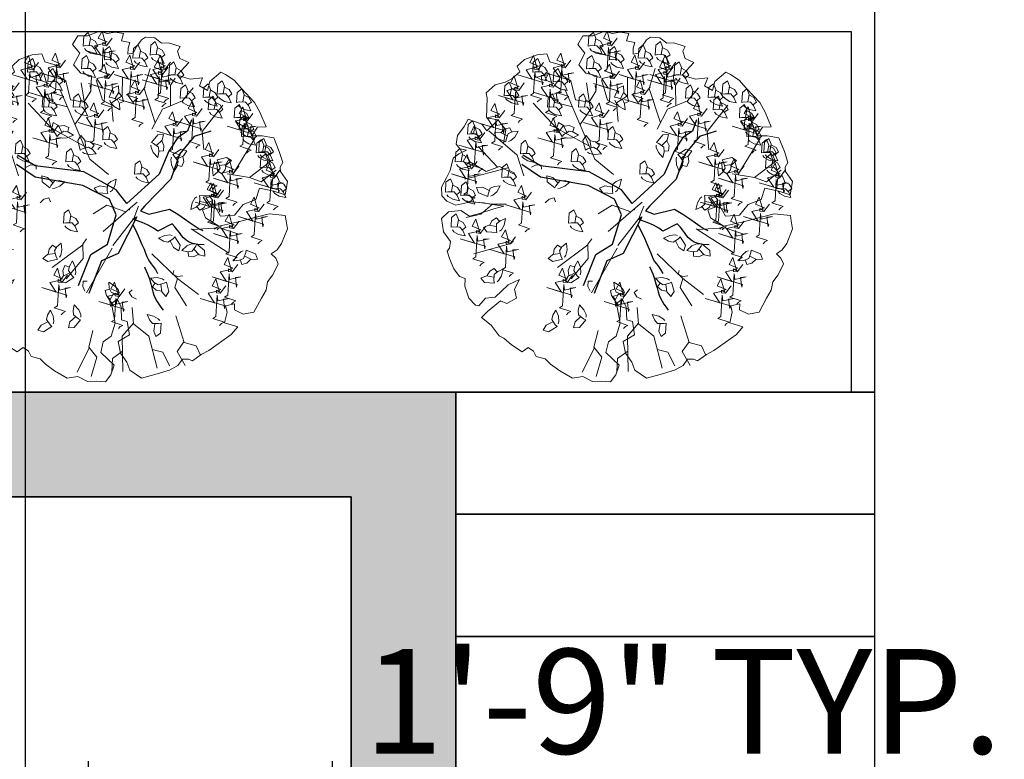
# Model space of a CAD drawing. Units: inches. Extents: x 2831 to 4250, y 1103 to 1797.
# Tile 12 of 15: x 3730 to 3814, y 1658 to 1722. Entities that reach past the tile are written whole.
import ezdxf

# ---------------------------------------------------------------- set-up
doc = ezdxf.new("R2010")
doc.units = ezdxf.units.IN
for name, color, linetype, lineweight in [('A-ANNO-DIMS', 2, 'Continuous', 18), ('A-WALL', 7, 'Continuous', 35), ('A-WALL-PATT', 252, 'Continuous', 13), ('ARBOL', 30, 'Continuous', 13), ('C-PROP', 7, 'Continuous', 25)]:
    doc.layers.add(name, color=color, linetype=linetype, lineweight=lineweight)
doc.layers.add('TALLO', color=36, linetype='Continuous')
doc.styles.get("Standard").update_dxf_attribs({"font": 'arial.ttf'})
doc.dimstyles.new('ISO-25', dxfattribs={"dimtxt": 9, "dimasz": 2.5, "dimexe": 1.25, "dimexo": 0.625, "dimtad": 1, "dimdec": 1, "dimlunit": 3, "dimtxsty": 'Standard', "dimcen": 2.5, "dimadec": 0, "dimazin": 0, "dimtfac": 1, "dimtdec": 1, "dimtmove": 0, "dimatfit": 3, "dimfxl": 1, "dimarcsym": 0})

# ---------------------------------------------------------------- blocks, each defined once
blk = doc.blocks.new('fresno')
at = {"layer": 'ARBOL'}
for p, q in [((2.96, 0.991), (3.575, 1.984)), ((-3.638, 1.194), (-4.164, 1.76)), ((-1.151, -0.932), (-1.99, -1.556)), ((-0.974, -3.757), (-1.31, -4.423))]:
    blk.add_line(p, q, dxfattribs=at)
blk.add_lwpolyline([(0.823, 4.745), (0.566, 4.764), (0.459, 4.687), (0.336, 4.518), (0.233, 4.322), (0.087, 4.298), (0.091, 4.464), (0.14, 4.621), (-0.09, 4.659), (-0.033, 4.863), (-0.264, 4.901), (-0.483, 4.866), (-0.686, 4.924), (-1.021, 4.801), (-1.288, 4.8), (-1.431, 4.563), (-1.234, 4.327), (-1.406, 4), (-1.205, 3.778), (-0.909, 3.705), (-0.931, 3.283), (-1.122, 2.983), (-1.491, 3.043), (-1.619, 3.562), (-1.9, 3.727), (-1.851, 3.982), (-2.197, 4.084), (-2.278, 4.31), (-2.543, 4.283), (-2.896, 4.152), (-3.091, 3.971), (-3.022, 3.817), (-3.244, 3.617), (-3.424, 3.528), (-3.697, 3.455), (-3.946, 3.236), (-3.922, 3.09), (-3.94, 2.548), (-3.617, 2.495), (-3.927, 2.19), (-4.062, 2.379), (-4.443, 2.512), (-4.546, 2.316), (-4.73, 2.062), (-4.767, 1.832), (-4.671, 1.698), (-4.486, 1.667), (-4.693, 1.559), (-4.854, 1.444), (-4.934, 1.102), (-5.037, 0.905), (-5.175, 0.644), (-5.166, 0.406), (-5.024, 0.264), (-4.781, 0.153), (-4.363, 0.249), (-4.014, 0.215), (-3.783, 0.177), (-3.46, 0.124), (-3.733, 0.051), (-4.132, -0.073), (-4.404, -0.146), (-4.639, 0.011), (-4.977, -0.028), (-5.172, -0.209), (-5.113, -0.574), (-4.921, -0.843), (-4.951, -1.027), (-5.012, -1.112), (-4.95, -1.311), (-4.83, -1.592), (-4.676, -1.807), (-4.518, -1.856), (-4.529, -2.068), (-4.417, -2.394), (-4.236, -2.59), (-4.143, -2.605), (-3.967, -2.397), (-3.703, -2.37), (-3.339, -2.027), (-3.032, -1.889), (-3.169, -2.15), (-3.115, -2.396), (-3.376, -2.542), (-3.552, -2.466), (-3.909, -2.762), (-4.077, -2.924), (-3.804, -3.135), (-3.592, -3.43), (-3.461, -3.499), (-3.253, -3.676), (-2.953, -3.867), (-2.792, -3.752), (-2.642, -3.848), (-2.572, -4.001), (-2.323, -4.066), (-2.18, -4.208), (-1.926, -4.392), (-1.58, -4.591), (-1.288, -4.545), (-1.027, -4.683), (-0.788, -4.675), (-0.531, -4.693), (-0.382, -4.505), (-0.29, -4.236), (-0.66, -3.891), (-0.588, -3.595), (-0.374, -3.441), (-0.267, -3.079), (-0.368, -2.541), (-0.208, -2.426), (-0.099, -2.633), (-0.087, -2.991), (0.071, -3.04), (0.129, -3.405), (-0.185, -3.59), (-0.119, -3.909), (0.055, -4.151), (0.136, -4.377), (0.456, -4.596), (0.828, -4.491), (1.227, -4.368), (1.461, -4.241), (1.583, -4.071), (1.748, -4.075), (1.86, -4.117), (2.101, -3.944), (2.308, -3.836), (2.925, -3.393), (3.101, -3.185), (2.74, -3.078), (2.812, -2.782), (2.769, -2.61), (3.015, -2.555), (3.012, -2.721), (3.254, -2.832), (3.546, -2.785), (3.752, -2.393), (3.882, -2.177), (3.92, -1.947), (4.069, -1.758), (4.214, -1.451), (4.144, -1.297), (4.021, -1.182), (4.182, -1.067), (4.304, -0.897), (4.464, -0.497), (4.429, -0.279), (4.406, -0.133), (3.964, -0.083), (3.074, -0.315), (2.582, -0.424), (2.217, -0.197), (2.136, 0.029), (2.462, 0.141), (2.628, -0.147), (3.012, -0.116), (3.249, 0.177), (3.602, 0.308), (3.701, 0.623), (4.089, 0.535), (4.404, 0.436), (4.464, 0.805), (4.272, 1.074), (4.267, 1.193), (4.336, 1.324), (4.243, 1.623), (4.092, 2.003), (3.769, 2.057), (3.485, 2.056), (3.642, 2.291), (3.88, 2.299), (3.71, 2.706), (3.563, 2.967), (3.201, 3.358), (3.001, 3.581), (2.766, 3.738), (2.635, 3.807), (2.332, 3.549), (2.268, 3.299), (2.052, 3.429), (2.136, 3.652), (1.798, 3.613), (1.437, 3.72), (1.755, 4.071), (1.513, 4.182), (1.451, 4.381), (1.519, 4.512), (1.204, 4.611), (1.012, 4.596)], close=True, dxfattribs=at)
for points in [[(-1.104, 4.45), (-1.063, 4.399), (-0.939, 4.325), (-0.757, 4.285), (-0.82, 4.431), (-0.903, 4.527), (-1.075, 4.533), (-1.143, 4.521), (-1.126, 4.792), (-1.002, 4.891), (-0.939, 4.738), (-0.975, 4.535)], [(-0.346, 4.735), (-0.501, 4.528), (-0.605, 4.545), (-0.605, 4.614), (-0.519, 4.563), (-0.622, 4.925), (-0.726, 4.735), (-0.484, 4.632), (-0.622, 4.58), (-0.829, 4.528), (-0.657, 4.27), (-1.053, 4.39), (-0.363, 4.183), (-0.381, 4.114), (-0.415, 4.373), (-0.26, 4.39), (-0.57, 4.321), (-0.588, 4.476), (-0.622, 3.89), (-0.708, 3.839), (-0.398, 3.735), (-0.467, 3.701), (-0.519, 3.649)], [(-0.935, 4.717), (-0.809, 4.65), (-0.736, 4.529), (-0.824, 4.459)], [(0.734, 4.203), (0.775, 4.152), (0.9, 4.078), (1.082, 4.038), (1.018, 4.185), (0.936, 4.281), (0.763, 4.287), (0.696, 4.274), (0.712, 4.546), (0.837, 4.645), (0.899, 4.491), (0.863, 4.289)], [(-0.521, 4.069), (-0.48, 4.018), (-0.356, 3.944), (-0.174, 3.904), (-0.237, 4.051), (-0.32, 4.146), (-0.492, 4.152), (-0.56, 4.14), (-0.543, 4.411), (-0.419, 4.511), (-0.356, 4.357), (-0.392, 4.154)], [(-0.352, 4.337), (-0.226, 4.269), (-0.153, 4.148), (-0.241, 4.078)], [(0.263, 4.114), (0.304, 4.063), (0.429, 3.989), (0.611, 3.948), (0.547, 4.095), (0.465, 4.191), (0.293, 4.197), (0.225, 4.185), (0.242, 4.456), (0.366, 4.555), (0.428, 4.402), (0.393, 4.199)], [(0.433, 4.381), (0.558, 4.314), (0.631, 4.193), (0.544, 4.122)], [(0.904, 4.471), (1.029, 4.404), (1.102, 4.282), (1.015, 4.212)], [(-2.368, 4.073), (-2.523, 3.866), (-2.627, 3.883), (-2.627, 3.952), (-2.541, 3.9), (-2.644, 4.262), (-2.748, 4.073), (-2.506, 3.969), (-2.644, 3.918), (-2.851, 3.866), (-2.679, 3.607), (-3.075, 3.728), (-2.385, 3.521), (-2.403, 3.452), (-2.437, 3.711), (-2.282, 3.728), (-2.592, 3.659), (-2.61, 3.814), (-2.644, 3.228), (-2.73, 3.176), (-2.42, 3.073), (-2.489, 3.038), (-2.541, 2.987)], [(-2.629, 3.733), (-2.588, 3.682), (-2.463, 3.608), (-2.281, 3.568), (-2.345, 3.715), (-2.427, 3.81), (-2.6, 3.816), (-2.667, 3.804), (-2.651, 4.075), (-2.526, 4.175), (-2.464, 4.021), (-2.5, 3.818)], [(-1.623, 4.132), (-1.778, 3.925), (-1.882, 3.942), (-1.882, 4.011), (-1.795, 3.959), (-1.899, 4.321), (-2.002, 4.132), (-1.761, 4.028), (-1.899, 3.977), (-2.106, 3.925), (-1.933, 3.666), (-2.33, 3.787), (-1.64, 3.58), (-1.657, 3.511), (-1.692, 3.77), (-1.537, 3.787), (-1.847, 3.718), (-1.864, 3.873), (-1.899, 3.287), (-1.985, 3.235), (-1.675, 3.132), (-1.744, 3.097), (-1.795, 3.046)], [(-1.149, 3.822), (-1.108, 3.771), (-0.983, 3.697), (-0.802, 3.657), (-0.865, 3.804), (-0.948, 3.9), (-1.12, 3.906), (-1.188, 3.893), (-1.171, 4.165), (-1.047, 4.264), (-0.984, 4.111), (-1.02, 3.908)], [(-0.98, 4.09), (-0.854, 4.023), (-0.781, 3.901), (-0.869, 3.831)], [(0.413, 4.08), (0.258, 3.873), (0.154, 3.89), (0.154, 3.959), (0.241, 3.908), (0.137, 4.27), (0.034, 4.08), (0.275, 3.977), (0.137, 3.925), (-0.07, 3.873), (0.103, 3.614), (-0.294, 3.735), (0.396, 3.528), (0.379, 3.459), (0.344, 3.718), (0.499, 3.735), (0.189, 3.666), (0.172, 3.821), (0.137, 3.235), (0.051, 3.183), (0.361, 3.08), (0.292, 3.046), (0.241, 2.994)], [(1.189, 3.942), (1.034, 3.735), (0.931, 3.752), (0.931, 3.821), (1.017, 3.77), (0.913, 4.132), (0.81, 3.942), (1.051, 3.839), (0.913, 3.787), (0.706, 3.735), (0.879, 3.477), (0.482, 3.597), (1.172, 3.39), (1.155, 3.321), (1.12, 3.58), (1.276, 3.597), (0.965, 3.528), (0.948, 3.683), (0.913, 3.097), (0.827, 3.046), (1.138, 2.942), (1.069, 2.908), (1.017, 2.856)], [(1.259, 4.08), (1.103, 3.873), (1, 3.89), (1, 3.959), (1.086, 3.908), (0.982, 4.27), (0.879, 4.08), (1.12, 3.977), (0.982, 3.925), (0.775, 3.873), (0.948, 3.614), (0.551, 3.735), (1.241, 3.528), (1.224, 3.459), (1.189, 3.718), (1.345, 3.735), (1.034, 3.666), (1.017, 3.821), (0.982, 3.235), (0.896, 3.183), (1.207, 3.08), (1.138, 3.046), (1.086, 2.994)], [(1.25, 3.643), (1.291, 3.592), (1.416, 3.518), (1.597, 3.478), (1.534, 3.625), (1.451, 3.721), (1.279, 3.727), (1.211, 3.714), (1.228, 3.985), (1.352, 4.085), (1.415, 3.931), (1.379, 3.729)], [(-1.951, 3.597), (-2.106, 3.39), (-2.209, 3.408), (-2.209, 3.477), (-2.123, 3.425), (-2.227, 3.787), (-2.33, 3.597), (-2.089, 3.494), (-2.227, 3.442), (-2.434, 3.39), (-2.261, 3.132), (-2.658, 3.252), (-1.968, 3.046), (-1.985, 2.977), (-2.02, 3.235), (-1.864, 3.252), (-2.175, 3.183), (-2.192, 3.339), (-2.227, 2.752), (-2.313, 2.701), (-2.002, 2.597), (-2.071, 2.563), (-2.123, 2.511)], [(-2.459, 4), (-2.334, 3.933), (-2.261, 3.812), (-2.348, 3.742)], [(-2.068, 3.464), (-2.027, 3.413), (-1.903, 3.339), (-1.721, 3.299), (-1.784, 3.446), (-1.867, 3.542), (-2.039, 3.547), (-2.107, 3.535), (-2.09, 3.806), (-1.966, 3.906), (-1.903, 3.752), (-1.939, 3.55)], [(-0.287, 3.833), (-0.442, 3.626), (-0.546, 3.643), (-0.546, 3.712), (-0.46, 3.661), (-0.563, 4.023), (-0.667, 3.833), (-0.425, 3.73), (-0.563, 3.678), (-0.77, 3.626), (-0.598, 3.367), (-0.995, 3.488), (-0.304, 3.281), (-0.322, 3.212), (-0.356, 3.471), (-0.201, 3.488), (-0.511, 3.419), (-0.529, 3.574), (-0.563, 2.988), (-0.649, 2.936), (-0.339, 2.833), (-0.408, 2.799), (-0.46, 2.747)], [(0.837, 2.414), (0.533, 3.352), (0.697, 3.906)], [(1.419, 3.911), (1.545, 3.844), (1.618, 3.722), (1.53, 3.652)], [(-2.898, 3.511), (-3.053, 3.304), (-3.157, 3.321), (-3.157, 3.39), (-3.071, 3.339), (-3.174, 3.701), (-3.278, 3.511), (-3.036, 3.408), (-3.174, 3.356), (-3.381, 3.304), (-3.209, 3.046), (-3.605, 3.166), (-2.915, 2.959), (-2.932, 2.89), (-2.967, 3.149), (-2.812, 3.166), (-3.122, 3.097), (-3.14, 3.253), (-3.174, 2.666), (-3.26, 2.615), (-2.95, 2.511), (-3.019, 2.477), (-3.071, 2.425)], [(-3.413, 3.083), (-3.373, 3.032), (-3.248, 2.958), (-3.066, 2.918), (-3.129, 3.065), (-3.212, 3.161), (-3.384, 3.167), (-3.452, 3.154), (-3.435, 3.425), (-3.311, 3.525), (-3.248, 3.371), (-3.284, 3.169)], [(-1.899, 3.732), (-1.773, 3.664), (-1.7, 3.543), (-1.788, 3.473)], [(-0.358, 2.895), (-0.615, 3.037), (-0.783, 3.596)], [(-0.063, 3.671), (-0.069, 3.151), (-0.364, 2.965), (-0.319, 2.449)], [(0.558, 3.402), (0.403, 3.195), (0.299, 3.212), (0.299, 3.281), (0.386, 3.23), (0.282, 3.592), (0.179, 3.402), (0.42, 3.299), (0.282, 3.247), (0.075, 3.195), (0.248, 2.936), (-0.149, 3.057), (0.541, 2.85), (0.524, 2.781), (0.489, 3.04), (0.644, 3.057), (0.334, 2.988), (0.317, 3.143), (0.282, 2.557), (0.196, 2.505), (0.506, 2.402), (0.437, 2.368), (0.386, 2.316)], [(1.259, 2.882), (1.254, 3.446), (1.381, 3.636)], [(2.573, 3.128), (2.613, 3.077), (2.738, 3.003), (2.92, 2.963), (2.857, 3.11), (2.774, 3.205), (2.602, 3.211), (2.534, 3.199), (2.551, 3.47), (2.675, 3.57), (2.738, 3.416), (2.702, 3.214)], [(-3.244, 3.351), (-3.118, 3.284), (-3.045, 3.162), (-3.133, 3.092)], [(-0.448, 1), (-0.961, 1.419), (-1.784, 3.341)], [(-1.367, 2.367), (-1.081, 2.78), (-1.193, 3.514)], [(-0.923, 3.449), (-0.951, 3.425), (-0.93, 3.313)], [(-0.41, 3.035), (-0.387, 2.974), (-0.291, 2.865), (-0.131, 2.771), (-0.146, 2.93), (-0.195, 3.047), (-0.357, 3.106), (-0.425, 3.115), (-0.325, 3.368), (-0.176, 3.424), (-0.164, 3.258), (-0.261, 3.077)], [(0.746, 2.242), (1.034, 2.786), (1.584, 3.019), (1.879, 3.374)], [(1.564, 3.016), (1.605, 2.965), (1.729, 2.891), (1.911, 2.851), (1.848, 2.998), (1.765, 3.094), (1.593, 3.099), (1.525, 3.087), (1.542, 3.358), (1.666, 3.458), (1.729, 3.304), (1.693, 3.102)], [(1.733, 3.284), (1.859, 3.216), (1.932, 3.095), (1.844, 3.025)], [(2.191, 3.038), (2.232, 2.987), (2.357, 2.913), (2.539, 2.873), (2.475, 3.02), (2.393, 3.116), (2.221, 3.122), (2.153, 3.109), (2.17, 3.381), (2.294, 3.48), (2.356, 3.326), (2.321, 3.124)], [(2.361, 3.306), (2.486, 3.239), (2.559, 3.117), (2.472, 3.047)], [(2.742, 3.396), (2.868, 3.328), (2.941, 3.207), (2.853, 3.137)], [(3.111, 2.904), (3.152, 2.853), (3.276, 2.779), (3.458, 2.739), (3.395, 2.886), (3.312, 2.981), (3.14, 2.987), (3.072, 2.975), (3.089, 3.246), (3.213, 3.346), (3.276, 3.192), (3.24, 2.99)], [(-2.225, 2.77), (-2.184, 2.718), (-2.06, 2.645), (-1.878, 2.604), (-1.941, 2.751), (-2.024, 2.847), (-2.196, 2.853), (-2.264, 2.84), (-2.247, 3.112), (-2.123, 3.211), (-2.06, 3.058), (-2.096, 2.855)], [(-1.575, 2.854), (-2.052, 2.969), (-2.2, 3.178)], [(-2.056, 3.037), (-1.93, 2.97), (-1.857, 2.849), (-1.945, 2.778)], [(-1.373, 2.77), (-1.332, 2.718), (-1.208, 2.645), (-1.026, 2.604), (-1.089, 2.751), (-1.172, 2.847), (-1.344, 2.853), (-1.412, 2.84), (-1.395, 3.112), (-1.271, 3.211), (-1.208, 3.058), (-1.244, 2.855)], [(-1.204, 3.037), (-1.078, 2.97), (-1.005, 2.849), (-1.093, 2.778)], [(-0.166, 3.238), (-0.068, 3.135), (-0.036, 2.997), (-0.141, 2.957)], [(2.121, 2.804), (1.966, 2.597), (1.862, 2.615), (1.862, 2.683), (1.949, 2.632), (1.845, 2.994), (1.742, 2.804), (1.983, 2.701), (1.845, 2.649), (1.638, 2.597), (1.811, 2.339), (1.414, 2.459), (2.104, 2.252), (2.087, 2.184), (2.052, 2.442), (2.207, 2.459), (1.897, 2.39), (1.88, 2.546), (1.845, 1.959), (1.759, 1.908), (2.069, 1.804), (2, 1.77), (1.949, 1.718)], [(2.326, 2.702), (2.367, 2.651), (2.492, 2.577), (2.673, 2.537), (2.61, 2.684), (2.527, 2.78), (2.355, 2.786), (2.287, 2.773), (2.304, 3.045), (2.428, 3.144), (2.491, 2.99), (2.455, 2.788)], [(3.28, 3.172), (3.406, 3.104), (3.479, 2.983), (3.391, 2.913)], [(-3.434, 2.752), (-3.59, 2.546), (-3.693, 2.563), (-3.693, 2.632), (-3.607, 2.58), (-3.71, 2.942), (-3.814, 2.752), (-3.572, 2.649), (-3.71, 2.597), (-3.917, 2.546), (-3.745, 2.287), (-4.142, 2.408), (-3.452, 2.201), (-3.469, 2.132), (-3.503, 2.39), (-3.348, 2.408), (-3.659, 2.339), (-3.676, 2.494), (-3.71, 1.908), (-3.797, 1.856), (-3.486, 1.753), (-3.555, 1.718), (-3.607, 1.666)], [(-1.112, 1.773), (-2.014, 2.265), (-2.654, 2.957)], [(-0.57, 2.77), (-0.726, 2.563), (-0.829, 2.58), (-0.829, 2.649), (-0.743, 2.597), (-0.846, 2.959), (-0.95, 2.77), (-0.708, 2.666), (-0.846, 2.615), (-1.053, 2.563), (-0.881, 2.304), (-1.278, 2.425), (-0.588, 2.218), (-0.605, 2.149), (-0.639, 2.408), (-0.484, 2.425), (-0.795, 2.356), (-0.812, 2.511), (-0.846, 1.925), (-0.933, 1.873), (-0.622, 1.77), (-0.691, 1.735), (-0.743, 1.684)], [(1.586, 2.528), (1.431, 2.321), (1.327, 2.339), (1.327, 2.408), (1.414, 2.356), (1.31, 2.718), (1.207, 2.528), (1.448, 2.425), (1.31, 2.373), (1.103, 2.321), (1.276, 2.063), (0.879, 2.184), (1.569, 1.977), (1.552, 1.908), (1.517, 2.166), (1.673, 2.184), (1.362, 2.115), (1.345, 2.27), (1.31, 1.684), (1.224, 1.632), (1.535, 1.528), (1.466, 1.494), (1.414, 1.442)], [(2.171, 1.674), (2.121, 2.172), (2.689, 2.898)], [(2.495, 2.97), (2.621, 2.903), (2.694, 2.781), (2.606, 2.711)], [(3.519, 2.666), (3.363, 2.459), (3.26, 2.477), (3.26, 2.546), (3.346, 2.494), (3.243, 2.856), (3.139, 2.666), (3.381, 2.563), (3.243, 2.511), (3.036, 2.459), (3.208, 2.201), (2.811, 2.321), (3.501, 2.115), (3.484, 2.046), (3.45, 2.304), (3.605, 2.321), (3.294, 2.252), (3.277, 2.408), (3.243, 1.821), (3.156, 1.77), (3.467, 1.666), (3.398, 1.632), (3.346, 1.58)], [(3.043, 2.478), (3.084, 2.427), (3.209, 2.353), (3.391, 2.313), (3.327, 2.46), (3.245, 2.556), (3.073, 2.562), (3.005, 2.549), (3.022, 2.82), (3.146, 2.92), (3.208, 2.766), (3.173, 2.564)], [(3.213, 2.746), (3.338, 2.679), (3.411, 2.557), (3.324, 2.487)], [(-4.422, 2.03), (-4.381, 1.979), (-4.257, 1.905), (-4.075, 1.865), (-4.138, 2.012), (-4.221, 2.108), (-4.393, 2.114), (-4.461, 2.101), (-4.444, 2.372), (-4.32, 2.472), (-4.257, 2.318), (-4.293, 2.116)], [(-3.468, 1.85), (-3.409, 2.222), (-3.628, 2.505)], [(-1.817, 2.351), (-1.972, 2.144), (-2.075, 2.162), (-2.075, 2.231), (-1.989, 2.179), (-2.093, 2.541), (-2.196, 2.351), (-1.955, 2.248), (-2.093, 2.196), (-2.3, 2.144), (-2.127, 1.886), (-2.524, 2.006), (-1.834, 1.8), (-1.851, 1.731), (-1.886, 1.989), (-1.73, 2.006), (-2.041, 1.937), (-2.058, 2.093), (-2.093, 1.506), (-2.179, 1.455), (-1.868, 1.351), (-1.937, 1.317), (-1.989, 1.265)], [(3.178, 2.165), (3.219, 2.113), (3.344, 2.04), (3.525, 1.999), (3.462, 2.146), (3.379, 2.242), (3.207, 2.248), (3.139, 2.236), (3.156, 2.507), (3.28, 2.606), (3.343, 2.453), (3.307, 2.25)], [(-3.986, 2.149), (-4.142, 1.942), (-4.245, 1.959), (-4.245, 2.028), (-4.159, 1.977), (-4.262, 2.339), (-4.366, 2.149), (-4.124, 2.046), (-4.262, 1.994), (-4.47, 1.942), (-4.297, 1.684), (-4.694, 1.804), (-4.004, 1.597), (-4.021, 1.528), (-4.055, 1.787), (-3.9, 1.804), (-4.211, 1.735), (-4.228, 1.89), (-4.262, 1.304), (-4.349, 1.253), (-4.038, 1.149), (-4.107, 1.115), (-4.159, 1.063)], [(-4.253, 2.298), (-4.127, 2.231), (-4.054, 2.109), (-4.142, 2.039)], [(-2.916, 0.958), (-3.096, 1.528), (-3.871, 2.197)], [(-3.331, 1.905), (-3.269, 1.928), (-3.161, 2.024), (-3.066, 2.184), (-3.226, 2.169), (-3.342, 2.121), (-3.401, 1.958), (-3.41, 1.89), (-3.663, 1.99), (-3.719, 2.139), (-3.554, 2.151), (-3.372, 2.054)], [(-3.533, 2.149), (-3.43, 2.247), (-3.292, 2.279), (-3.252, 2.174)], [(-1.786, 2.007), (-1.722, 1.99), (-1.578, 2.003), (-1.407, 2.078), (-1.545, 2.159), (-1.668, 2.188), (-1.811, 2.092), (-1.859, 2.042), (-2.004, 2.271), (-1.962, 2.425), (-1.821, 2.337), (-1.731, 2.152)], [(-1.806, 2.323), (-1.665, 2.343), (-1.534, 2.287), (-1.564, 2.179)], [(-0.566, 1.873), (-0.525, 1.822), (-0.4, 1.748), (-0.219, 1.708), (-0.282, 1.855), (-0.365, 1.951), (-0.537, 1.957), (-0.605, 1.944), (-0.588, 2.216), (-0.464, 2.315), (-0.401, 2.162), (-0.437, 1.959)], [(3.245, 1.963), (3.286, 1.912), (3.411, 1.838), (3.593, 1.798), (3.529, 1.945), (3.447, 2.041), (3.274, 2.046), (3.206, 2.034), (3.223, 2.305), (3.347, 2.405), (3.41, 2.251), (3.374, 2.049)], [(3.347, 2.432), (3.473, 2.365), (3.546, 2.244), (3.458, 2.173)], [(3.415, 2.231), (3.54, 2.163), (3.613, 2.042), (3.525, 1.972)], [(-2.965, 1.493), (-2.924, 1.441), (-2.799, 1.368), (-2.618, 1.327), (-2.681, 1.474), (-2.764, 1.57), (-2.936, 1.576), (-3.004, 1.564), (-2.987, 1.835), (-2.863, 1.934), (-2.8, 1.781), (-2.836, 1.578)], [(-1.164, 1.612), (-1.109, 1.576), (-0.967, 1.544), (-0.782, 1.562), (-0.888, 1.682), (-0.996, 1.748), (-1.162, 1.7), (-1.222, 1.667), (-1.29, 1.93), (-1.203, 2.063), (-1.096, 1.937), (-1.067, 1.733)], [(-1.085, 1.919), (-0.945, 1.893), (-0.838, 1.801), (-0.9, 1.707)], [(-0.397, 2.141), (-0.271, 2.074), (-0.198, 1.952), (-0.286, 1.882)], [(0.72, 1.798), (0.723, 1.733), (0.781, 1.6), (0.904, 1.46), (0.939, 1.616), (0.929, 1.742), (0.793, 1.848), (0.73, 1.878), (0.904, 2.088), (1.062, 2.095), (1.023, 1.934), (0.875, 1.791)], [(1.014, 1.915), (1.077, 1.787), (1.064, 1.646), (0.952, 1.64)], [(3.649, 1.515), (3.69, 1.464), (3.814, 1.39), (3.996, 1.35), (3.933, 1.497), (3.85, 1.592), (3.678, 1.598), (3.61, 1.586), (3.627, 1.857), (3.751, 1.957), (3.814, 1.803), (3.778, 1.601)], [(3.716, 1.537), (3.757, 1.486), (3.882, 1.412), (4.063, 1.372), (4, 1.519), (3.917, 1.615), (3.745, 1.621), (3.677, 1.608), (3.694, 1.88), (3.818, 1.979), (3.881, 1.825), (3.845, 1.623)], [(-4.759, 1.269), (-4.718, 1.217), (-4.593, 1.144), (-4.411, 1.103), (-4.475, 1.25), (-4.557, 1.346), (-4.729, 1.352), (-4.797, 1.339), (-4.78, 1.611), (-4.656, 1.71), (-4.594, 1.557), (-4.629, 1.354)], [(-2.796, 1.76), (-2.67, 1.693), (-2.597, 1.572), (-2.685, 1.501)], [(-1.575, 1.269), (-1.534, 1.217), (-1.409, 1.144), (-1.228, 1.103), (-1.291, 1.25), (-1.373, 1.346), (-1.546, 1.352), (-1.614, 1.339), (-1.597, 1.611), (-1.473, 1.71), (-1.41, 1.557), (-1.446, 1.354)], [(1.283, 1.469), (1.266, 1.405), (1.279, 1.261), (1.354, 1.09), (1.435, 1.228), (1.464, 1.351), (1.368, 1.494), (1.318, 1.542), (1.547, 1.687), (1.7, 1.645), (1.613, 1.504), (1.428, 1.414)], [(2.587, 1.684), (2.432, 1.477), (2.328, 1.494), (2.328, 1.563), (2.414, 1.511), (2.311, 1.873), (2.207, 1.684), (2.449, 1.58), (2.311, 1.528), (2.104, 1.477), (2.276, 1.218), (1.88, 1.339), (2.57, 1.132), (2.552, 1.063), (2.518, 1.321), (2.673, 1.339), (2.363, 1.27), (2.345, 1.425), (2.311, 0.839), (2.225, 0.787), (2.535, 0.684), (2.466, 0.649), (2.414, 0.597)], [(3.818, 1.783), (3.944, 1.715), (4.017, 1.594), (3.929, 1.524)], [(3.885, 1.805), (4.011, 1.738), (4.084, 1.616), (3.996, 1.546)], [(-4.193, 1.356), (-4.349, 1.149), (-4.452, 1.166), (-4.452, 1.235), (-4.366, 1.184), (-4.469, 1.546), (-4.573, 1.356), (-4.331, 1.253), (-4.469, 1.201), (-4.677, 1.149), (-4.504, 0.89), (-4.901, 1.011), (-4.211, 0.804), (-4.228, 0.735), (-4.262, 0.994), (-4.107, 1.011), (-4.418, 0.942), (-4.435, 1.097), (-4.469, 0.511), (-4.556, 0.459), (-4.245, 0.356), (-4.314, 0.322), (-4.366, 0.27)], [(-4.589, 1.536), (-4.464, 1.469), (-4.391, 1.348), (-4.478, 1.277)], [(-1.406, 1.536), (-1.28, 1.469), (-1.207, 1.348), (-1.295, 1.277)], [(0.308, 0.933), (0.349, 0.881), (0.474, 0.807), (0.656, 0.767), (0.592, 0.914), (0.51, 1.01), (0.337, 1.016), (0.27, 1.003), (0.286, 1.275), (0.411, 1.374), (0.473, 1.221), (0.437, 1.018)], [(1.599, 1.489), (1.618, 1.348), (1.563, 1.217), (1.455, 1.247)], [(2.479, 1.34), (2.443, 1.285), (2.411, 1.143), (2.429, 0.958), (2.549, 1.064), (2.615, 1.172), (2.567, 1.338), (2.534, 1.398), (2.797, 1.466), (2.93, 1.379), (2.804, 1.272), (2.6, 1.243)], [(3.139, 1.235), (2.984, 1.028), (2.88, 1.046), (2.88, 1.115), (2.967, 1.063), (2.863, 1.425), (2.759, 1.235), (3.001, 1.132), (2.863, 1.08), (2.656, 1.028), (2.828, 0.77), (2.432, 0.891), (3.122, 0.684), (3.105, 0.615), (3.07, 0.873), (3.225, 0.891), (2.915, 0.822), (2.897, 0.977), (2.863, 0.391), (2.777, 0.339), (3.087, 0.235), (3.018, 0.201), (2.967, 0.149)], [(4.01, 1.36), (3.422, 0.918)], [(3.761, 1.112), (3.802, 1.061), (3.926, 0.987), (4.108, 0.947), (4.045, 1.093), (3.962, 1.189), (3.79, 1.195), (3.722, 1.183), (3.739, 1.454), (3.863, 1.553), (3.926, 1.4), (3.89, 1.197)], [(3.93, 1.379), (4.056, 1.312), (4.129, 1.191), (4.041, 1.121)], [(-3.354, 1.176), (-4.529, 0.864)], [(-3.192, 1.017), (-3.578, 1.215), (-3.949, 1.081), (-4.398, 1.339)], [(-3.481, 0.843), (-3.44, 0.792), (-3.315, 0.718), (-3.133, 0.678), (-3.197, 0.825), (-3.279, 0.92), (-3.451, 0.926), (-3.519, 0.914), (-3.502, 1.185), (-3.378, 1.285), (-3.316, 1.131), (-3.351, 0.928)], [(-3.311, 1.111), (-3.186, 1.043), (-3.113, 0.922), (-3.2, 0.852)], [(-2.703, 1.201), (-2.575, 1.263), (-2.433, 1.251), (-2.428, 1.139)], [(0.478, 1.2), (0.603, 1.133), (0.676, 1.011), (0.589, 0.941)], [(2.786, 1.261), (2.76, 1.121), (2.668, 1.014), (2.574, 1.076)], [(2.808, 1.015), (3.422, 0.918), (3.422, 0.918), (3.748, 0.794), (4.154, 1.111)], [(4.26, 1.115), (4.105, 0.908), (4.002, 0.925), (4.002, 0.994), (4.088, 0.942), (3.984, 1.304), (3.881, 1.115), (4.122, 1.011), (3.984, 0.959), (3.777, 0.908), (3.95, 0.649), (3.553, 0.77), (4.243, 0.563), (4.226, 0.494), (4.191, 0.753), (4.347, 0.77), (4.036, 0.701), (4.019, 0.856), (3.984, 0.27), (3.898, 0.218), (4.209, 0.115), (4.14, 0.08), (4.088, 0.029)], [(-5.028, 0.44), (-4.987, 0.388), (-4.862, 0.315), (-4.68, 0.274), (-4.744, 0.421), (-4.826, 0.517), (-4.998, 0.523), (-5.066, 0.511), (-5.049, 0.782), (-4.925, 0.881), (-4.863, 0.728), (-4.898, 0.525)], [(-1.981, 0.615), (-1.915, 0.618), (-1.782, 0.676), (-1.643, 0.799), (-1.799, 0.834), (-1.925, 0.824), (-2.031, 0.688), (-2.061, 0.626), (-2.27, 0.799), (-2.278, 0.958), (-2.117, 0.918), (-1.974, 0.77)], [(-0.397, 0.517), (-0.346, 0.557), (-0.272, 0.682), (-0.232, 0.864), (-0.379, 0.801), (-0.474, 0.718), (-0.48, 0.546), (-0.468, 0.478), (-0.739, 0.495), (-0.838, 0.619), (-0.685, 0.682), (-0.482, 0.646)], [(4.075, 0.529), (4.116, 0.478), (4.24, 0.404), (4.422, 0.364), (4.359, 0.511), (4.276, 0.607), (4.104, 0.613), (4.036, 0.6), (4.053, 0.871), (4.177, 0.971), (4.24, 0.817), (4.204, 0.615)], [(-4.858, 0.707), (-4.733, 0.64), (-4.66, 0.519), (-4.747, 0.448)], [(-4.602, 0.35), (-4.561, 0.299), (-4.436, 0.225), (-4.254, 0.185), (-4.318, 0.332), (-4.4, 0.428), (-4.572, 0.433), (-4.64, 0.421), (-4.623, 0.692), (-4.499, 0.792), (-4.437, 0.638), (-4.472, 0.436)], [(-4.432, 0.618), (-4.307, 0.55), (-4.234, 0.429), (-4.321, 0.359)], [(-3.824, 0.404), (-3.763, 0.427), (-3.654, 0.523), (-3.559, 0.683), (-3.719, 0.668), (-3.835, 0.62), (-3.894, 0.457), (-3.903, 0.389), (-4.156, 0.489), (-4.212, 0.638), (-4.047, 0.65), (-3.865, 0.553)], [(-2.698, 0.509), (-2.854, 0.302), (-2.957, 0.319), (-2.957, 0.388), (-2.871, 0.336), (-2.974, 0.698), (-3.078, 0.509), (-2.836, 0.405), (-2.974, 0.353), (-3.182, 0.302), (-3.009, 0.043), (-3.406, 0.164), (-2.716, -0.043), (-2.733, -0.112), (-2.767, 0.147), (-2.612, 0.164), (-2.923, 0.095), (-2.94, 0.25), (-2.974, -0.336), (-3.061, -0.388), (-2.75, -0.491), (-2.819, -0.526), (-2.871, -0.577)], [(2.639, 0.58), (2.483, 0.373), (2.38, 0.391), (2.38, 0.46), (2.466, 0.408), (2.363, 0.77), (2.259, 0.58), (2.501, 0.477), (2.363, 0.425), (2.156, 0.373), (2.328, 0.115), (1.931, 0.235), (2.621, 0.029), (2.604, -0.04), (2.57, 0.218), (2.725, 0.235), (2.414, 0.166), (2.397, 0.322), (2.363, -0.265), (2.276, -0.316), (2.587, -0.42), (2.518, -0.454), (2.466, -0.506)], [(2.708, 0.563), (2.552, 0.356), (2.449, 0.373), (2.449, 0.442), (2.535, 0.391), (2.432, 0.753), (2.328, 0.563), (2.57, 0.46), (2.432, 0.408), (2.225, 0.356), (2.397, 0.097), (2, 0.218), (2.69, 0.011), (2.673, -0.058), (2.639, 0.201), (2.794, 0.218), (2.483, 0.149), (2.466, 0.304), (2.432, -0.282), (2.345, -0.334), (2.656, -0.437), (2.587, -0.471), (2.535, -0.523)], [(4.244, 0.797), (4.37, 0.73), (4.443, 0.608), (4.355, 0.538)], [(-2.322, 0.222), (-2.219, 0.321), (-2.081, 0.353), (-2.042, 0.248)], [(1.978, 0.384), (1.927, 0.343), (1.853, 0.218), (1.813, 0.036), (1.96, 0.1), (2.056, 0.182), (2.061, 0.355), (2.049, 0.422), (2.32, 0.406), (2.42, 0.281), (2.266, 0.219), (2.064, 0.254)], [(3.829, 0.184), (3.674, -0.023), (3.57, -0.006), (3.57, 0.063), (3.657, 0.011), (3.553, 0.373), (3.45, 0.184), (3.691, 0.08), (3.553, 0.029), (3.346, -0.023), (3.519, -0.282), (3.122, -0.161), (3.812, -0.368), (3.795, -0.437), (3.76, -0.178), (3.915, -0.161), (3.605, -0.23), (3.588, -0.075), (3.553, -0.661), (3.467, -0.713), (3.777, -0.816), (3.708, -0.851), (3.657, -0.902)], [(-3.394, 0.18), (-3.77, 0.182), (-4.532, 0.27)], [(-3.77, 0.182), (-4.09, -0.088), (-4.494, -0.18)], [(-1.642, -0.412), (-1.601, -0.463), (-1.477, -0.537), (-1.295, -0.577), (-1.358, -0.43), (-1.441, -0.334), (-1.613, -0.328), (-1.681, -0.341), (-1.664, -0.069), (-1.54, 0.03), (-1.477, -0.124), (-1.513, -0.326)], [(0.03, -0.026), (-0.491, 0.154), (-0.871, -0.08)], [(-0.596, -0.564), (0.03, -0.026), (0.339, 0.235)], [(0.38, 0.131), (0.248, -0.21), (-0.33, -0.951)], [(2.246, 0.214), (2.178, 0.089), (2.057, 0.016), (1.987, 0.103)], [(-4.871, -0.524), (-4.83, -0.575), (-4.705, -0.649), (-4.523, -0.689), (-4.587, -0.542), (-4.669, -0.446), (-4.841, -0.44), (-4.909, -0.453), (-4.893, -0.181), (-4.768, -0.082), (-4.706, -0.236), (-4.741, -0.438)], [(-4.701, -0.256), (-4.576, -0.323), (-4.503, -0.445), (-4.59, -0.515)], [(-3.952, -0.42), (-4.107, -0.627), (-4.211, -0.609), (-4.211, -0.54), (-4.124, -0.592), (-4.228, -0.23), (-4.331, -0.42), (-4.09, -0.523), (-4.228, -0.575), (-4.435, -0.627), (-4.262, -0.885), (-4.659, -0.765), (-3.969, -0.971), (-3.986, -1.04), (-4.021, -0.782), (-3.866, -0.765), (-4.176, -0.834), (-4.193, -0.678), (-4.228, -1.265), (-4.314, -1.316), (-4.004, -1.42), (-4.073, -1.454), (-4.124, -1.506)], [(-3.58, -0.559), (-3.529, -0.518), (-3.455, -0.393), (-3.415, -0.211), (-3.562, -0.275), (-3.658, -0.357), (-3.664, -0.53), (-3.651, -0.597), (-3.923, -0.581), (-4.022, -0.456), (-3.868, -0.394), (-3.666, -0.43)], [(-3.848, -0.389), (-3.781, -0.264), (-3.659, -0.191), (-3.589, -0.278)], [(-1.473, -0.144), (-1.347, -0.211), (-1.274, -0.333), (-1.362, -0.403)], [(3.139, -0.282), (2.984, -0.489), (2.88, -0.471), (2.88, -0.402), (2.967, -0.454), (2.863, -0.092), (2.759, -0.282), (3.001, -0.385), (2.863, -0.437), (2.656, -0.489), (2.828, -0.747), (2.432, -0.627), (3.122, -0.834), (3.105, -0.902), (3.07, -0.644), (3.225, -0.627), (2.915, -0.696), (2.897, -0.54), (2.863, -1.127), (2.777, -1.178), (3.087, -1.282), (3.018, -1.316), (2.967, -1.368)], [(-3.141, -0.713), (-3.296, -0.92), (-3.4, -0.902), (-3.4, -0.834), (-3.314, -0.885), (-3.417, -0.523), (-3.521, -0.713), (-3.279, -0.816), (-3.417, -0.868), (-3.624, -0.92), (-3.452, -1.178), (-3.848, -1.058), (-3.158, -1.265), (-3.175, -1.333), (-3.21, -1.075), (-3.055, -1.058), (-3.365, -1.127), (-3.383, -0.971), (-3.417, -1.558), (-3.503, -1.609), (-3.193, -1.713), (-3.262, -1.747), (-3.314, -1.799)], [(1.822, -0.495), (2.859, -1.165)], [(1.846, -0.51), (2.605, -0.469), (3.129, -0.637)], [(-1.047, -0.767), (-1.151, -0.913), (-1.144, -1.307), (-1.61, -1.871)], [(1.304, -0.681), (1.241, -0.664), (1.097, -0.678), (0.926, -0.752), (1.064, -0.833), (1.187, -0.862), (1.33, -0.766), (1.377, -0.716), (1.523, -0.945), (1.481, -1.099), (1.34, -1.011), (1.25, -0.826)], [(-3.195, -0.824), (-3.267, -0.898), (-4.285, -1.185)], [(-1.794, -1.268), (-1.758, -1.214), (-1.726, -1.072), (-1.744, -0.887), (-1.865, -0.993), (-1.93, -1.101), (-1.883, -1.266), (-1.85, -1.327), (-2.113, -1.395), (-2.246, -1.307), (-2.119, -1.2), (-1.916, -1.172)], [(-2.101, -1.19), (-2.076, -1.05), (-1.983, -0.943), (-1.889, -1.004)], [(-0.346, -1.024), (-1.05, -2.251)], [(1.903, -0.903), (1.837, -0.905), (1.704, -0.963), (1.565, -1.086), (1.721, -1.122), (1.847, -1.111), (1.953, -0.975), (1.983, -0.913), (2.192, -1.086), (2.2, -1.245), (2.039, -1.205), (1.896, -1.057)], [(3.253, -1.094), (3.192, -1.117), (3.083, -1.213), (2.988, -1.374), (3.148, -1.359), (3.264, -1.31), (3.323, -1.148), (3.332, -1.079), (3.585, -1.179), (3.641, -1.328), (3.476, -1.34), (3.294, -1.244)], [(0.748, -1.185), (1.452, -1.855), (2.021, -2.292)], [(2.02, -1.197), (1.891, -1.259), (1.75, -1.247), (1.745, -1.134)], [(3.105, -1.471), (2.949, -1.678), (2.846, -1.661), (2.846, -1.592), (2.932, -1.644), (2.829, -1.282), (2.725, -1.471), (2.967, -1.575), (2.829, -1.627), (2.621, -1.678), (2.794, -1.937), (2.397, -1.816), (3.087, -2.023), (3.07, -2.092), (3.036, -1.833), (3.191, -1.816), (2.88, -1.885), (2.863, -1.73), (2.829, -2.316), (2.742, -2.368), (3.053, -2.471), (2.984, -2.506), (2.932, -2.558)], [(3.455, -1.338), (3.352, -1.437), (3.214, -1.469), (3.175, -1.364)], [(-3.648, -1.948), (-3.596, -1.907), (-3.523, -1.782), (-3.482, -1.6), (-3.629, -1.664), (-3.725, -1.746), (-3.731, -1.919), (-3.719, -1.986), (-3.99, -1.97), (-4.089, -1.845), (-3.936, -1.783), (-3.733, -1.819)], [(-3.915, -1.778), (-3.848, -1.653), (-3.727, -1.58), (-3.656, -1.667)], [(-1.571, -1.764), (-1.726, -1.971), (-1.83, -1.954), (-1.83, -1.885), (-1.744, -1.937), (-1.847, -1.575), (-1.951, -1.764), (-1.709, -1.868), (-1.847, -1.92), (-2.054, -1.971), (-1.882, -2.23), (-2.278, -2.109), (-1.588, -2.316), (-1.605, -2.385), (-1.64, -2.127), (-1.485, -2.109), (-1.795, -2.178), (-1.813, -2.023), (-1.847, -2.609), (-1.933, -2.661), (-1.623, -2.764), (-1.692, -2.799), (-1.744, -2.851)], [(-1.361, -1.756), (-1.343, -1.693), (-1.357, -1.548), (-1.431, -1.377), (-1.513, -1.515), (-1.542, -1.638), (-1.445, -1.781), (-1.395, -1.829), (-1.625, -1.974), (-1.778, -1.932), (-1.691, -1.791), (-1.506, -1.701)], [(-1.677, -1.776), (-1.696, -1.635), (-1.641, -1.504), (-1.533, -1.534)], [(1.086, -1.899), (1.031, -1.863), (0.89, -1.831), (0.704, -1.849), (0.81, -1.969), (0.918, -2.035), (1.084, -1.987), (1.145, -1.954), (1.212, -2.218), (1.125, -2.35), (1.018, -2.224), (0.989, -2.02)], [(1.593, -1.781), (1.452, -1.801), (1.322, -1.746), (1.352, -1.637)], [(1.452, -1.855), (1.379, -2.105), (1.698, -2.609)], [(2.777, -2.058), (2.621, -2.264), (2.518, -2.247), (2.518, -2.178), (2.604, -2.23), (2.501, -1.868), (2.397, -2.058), (2.639, -2.161), (2.501, -2.213), (2.294, -2.264), (2.466, -2.523), (2.069, -2.402), (2.759, -2.609), (2.742, -2.678), (2.708, -2.42), (2.863, -2.402), (2.552, -2.471), (2.535, -2.316), (2.501, -2.902), (2.414, -2.954), (2.725, -3.057), (2.656, -3.092), (2.604, -3.144)], [(-1.092, -2.202), (-1.154, -2.074), (-1.142, -1.933), (-1.03, -1.928)], [(-0.001, -2.144), (-0.156, -2.351), (-0.26, -2.333), (-0.26, -2.264), (-0.174, -2.316), (-0.277, -1.954), (-0.381, -2.144), (-0.139, -2.247), (-0.277, -2.299), (-0.484, -2.351), (-0.312, -2.609), (-0.708, -2.489), (-0.018, -2.695), (-0.035, -2.764), (-0.07, -2.506), (0.085, -2.489), (-0.225, -2.558), (-0.243, -2.402), (-0.277, -2.989), (-0.363, -3.04), (-0.053, -3.144), (-0.122, -3.178), (-0.174, -3.23)], [(-0.405, -2.427), (-0.503, -2.324), (-0.535, -2.186), (-0.43, -2.146)], [(-0.161, -2.225), (-0.184, -2.163), (-0.28, -2.055), (-0.44, -1.96), (-0.425, -2.12), (-0.376, -2.236), (-0.214, -2.295), (-0.146, -2.304), (-0.246, -2.557), (-0.395, -2.613), (-0.407, -2.448), (-0.31, -2.266)], [(1.007, -2.206), (0.867, -2.181), (0.76, -2.088), (0.822, -1.994)], [(0.319, -2.428), (0.193, -2.361), (0.12, -2.239), (0.208, -2.169)], [(-1.201, -2.914), (-1.204, -2.849), (-1.262, -2.716), (-1.385, -2.576), (-1.42, -2.732), (-1.41, -2.858), (-1.274, -2.964), (-1.212, -2.994), (-1.385, -3.204), (-1.544, -3.211), (-1.504, -3.05), (-1.356, -2.907)], [(0.201, -2.655), (0.24, -3.105), (0.657, -3.436), (0.886, -4.322)], [(-1.966, -3.1), (-1.949, -3.037), (-1.962, -2.892), (-2.037, -2.722), (-2.118, -2.859), (-2.147, -2.982), (-2.051, -3.125), (-2.001, -3.173), (-2.23, -3.319), (-2.383, -3.277), (-2.296, -3.136), (-2.111, -3.046)], [(0.959, -3.012), (0.918, -2.961), (0.793, -2.887), (0.612, -2.847), (0.675, -2.994), (0.758, -3.089), (0.93, -3.095), (0.998, -3.083), (0.981, -3.354), (0.857, -3.453), (0.794, -3.3), (0.83, -3.097)], [(1.399, -2.886), (1.63, -3.612), (1.964, -3.708), (2.084, -3.964)], [(0.238, -3.084), (-0.067, -3.438), (-0.048, -4.412)], [(-0.923, -4.549), (-0.768, -4.012), (-0.99, -3.737), (-0.872, -3.28)], [(1.625, -3.596), (1.438, -3.858), (1.657, -4.248)], [(-0.059, -3.851), (-0.336, -4.054), (-0.355, -4.41)], [(0.752, -3.801), (1.042, -3.878), (1.233, -4.25)]]:
    blk.add_lwpolyline(points, dxfattribs=at)
for p in [(-0.308, 0.101), (0.124, 0.027)]:
    blk.add_point(p, dxfattribs=at)
at = {"layer": 'TALLO'}
for points in [[(1.829, 2.5), (1.722, 2.184), (1.454, 2.012), (1.213, 1.639), (0.944, 1.008), (0.06, 0.204), (-0.234, 0.577), (-1.119, 1.065), (-2.458, 1.237), (-2.941, 1.524)], [(2.364, 2.184), (1.909, 2.041), (1.507, 1.552), (1.266, 0.864), (0.542, 0.125), (0.433, 0.001), (0.662, -0.096), (1.228, 0.045), (1.455, -0.09), (1.644, -0.216), (1.8, -0.33), (1.931, -0.425), (2.042, -0.496), (2.141, -0.539)], [(-1.272, -2.047), (-0.931, -1.203), (-0.475, -0.916), (-0.234, -0.112), (-0.422, 0.318), (-1.146, 0.691), (-2.458, 0.921), (-2.967, 1.266)], [(2.177, -0.932), (2.008, -0.924), (1.873, -0.898), (1.766, -0.859), (1.682, -0.807), (1.613, -0.745), (1.554, -0.676), (1.499, -0.6), (1.442, -0.521), (1.376, -0.44), (1.298, -0.357), (0.908, -0.555), (0.791, -0.474), (0.647, -0.394), (0.474, -0.317), (0.265, -0.244), (0.226, -0.233), (0.328, -0.17), (-0.181, -1.175), (-0.637, -1.375), (-0.985, -2.265)], [(0.219, -0.386), (0.3, -0.544), (0.399, -0.753), (0.473, -0.922), (0.529, -1.057), (0.571, -1.164), (0.607, -1.251), (0.641, -1.324), (0.68, -1.389), (0.729, -1.454), (0.784, -1.525), (0.844, -1.61), (0.903, -1.717)], [(0.538, -1.536), (0.555, -1.568), (0.626, -1.728), (0.678, -1.871), (0.716, -2), (0.747, -2.115), (0.773, -2.219), (0.802, -2.314), (0.837, -2.401), (0.883, -2.483), (0.936, -2.562), (0.994, -2.642), (1.052, -2.727)]]:
    blk.add_lwpolyline(points, dxfattribs=at)
blk = doc.blocks.new('*D85')
at = {"layer": 'A-ANNO-DIMS', "color": 0, "lineweight": -2, "transparency": 16777216}
for p, q in [((3730.24, 1651.147), (3730.24, 1797.343)), ((3735.015, 1651.147), (3728.99, 1651.147)), ((3730.24, 1617.647), (3730.24, 1648.647)), ((3735.015, 1615.147), (3728.99, 1615.147))]:
    blk.add_line(p, q, dxfattribs=at)
at = {"layer": 'A-ANNO-DIMS', "color": 0, "transparency": 16777216}
for points in [[(3729.823, 1648.647), (3730.657, 1648.647), (3730.24, 1651.147)], [(3729.823, 1617.647), (3730.657, 1617.647), (3730.24, 1615.147)]]:
    blk.add_solid(points, dxfattribs=at)
at = {"layer": 'Defpoints', "color": 0, "transparency": 16777216}
for p in [(3730.24, 1651.147), (3735.64, 1651.147), (3735.64, 1615.147)]:
    blk.add_point(p, dxfattribs=at)
at = {"layer": 'A-ANNO-DIMS', "color": 0, "transparency": 16777216, "insert": (3724.955, 1725.495), "char_height": 9, "attachment_point": 5, "rotation": 90}
blk.add_mtext('DOUBLE SINK 3\'-0" TYP.', dxfattribs=at)
blk = doc.blocks.new('*D86')
at = {"layer": 'A-ANNO-DIMS', "color": 0, "lineweight": -2, "transparency": 16777216}
for p, q in [((3735.64, 1651.772), (3735.64, 1657.797)), ((3756.64, 1651.772), (3756.64, 1657.797)), ((3738.14, 1656.547), (3754.14, 1656.547)), ((3756.64, 1656.547), (3814.402, 1656.547))]:
    blk.add_line(p, q, dxfattribs=at)
at = {"layer": 'A-ANNO-DIMS', "color": 0, "transparency": 16777216}
for points in [[(3738.14, 1656.963), (3738.14, 1656.13), (3735.64, 1656.547)], [(3754.14, 1656.963), (3754.14, 1656.13), (3756.64, 1656.547)]]:
    blk.add_solid(points, dxfattribs=at)
at = {"layer": 'Defpoints', "color": 0, "transparency": 16777216}
for p in [(3756.64, 1656.547), (3735.64, 1651.147), (3756.64, 1651.147)]:
    blk.add_point(p, dxfattribs=at)
at = {"layer": 'A-ANNO-DIMS', "color": 0, "transparency": 16777216, "insert": (3786.771, 1661.767), "char_height": 9, "attachment_point": 5}
blk.add_mtext('1\'-9" TYP.', dxfattribs=at)

msp = doc.modelspace()

# ---------------------------------------------------------------- hatches: boundary and pattern name
at = {"layer": 'A-WALL-PATT'}
h = msp.add_hatch(color=256, dxfattribs=at)
h.dxf.hatch_style = 1
h.paths.add_polyline_path([(3783.227, 1560.513), (3767.227, 1560.513), (3767.227, 1572.513), (3761.227, 1572.513), (3758.227, 1572.513), (3758.227, 1560.513), (3488.227, 1560.513), (3488.227, 1562.513), (3485.227, 1562.513), (3479.227, 1562.513), (3479.227, 1552.513), (3485.227, 1552.513), (3488.227, 1552.513), (3488.227, 1554.513), (3642.227, 1554.513), (3642.227, 1498.513), (3648.227, 1498.513), (3648.227, 1554.513), (3720.227, 1554.513), (3720.227, 1498.513), (3726.227, 1498.513), (3726.227, 1554.513), (3774.227, 1554.513), (3774.227, 1528.513), (3783.227, 1528.513)])
h.paths.add_polyline_path([(3767.227, 1689.513), (3728.227, 1689.513), (3728.227, 1680.513), (3758.227, 1680.513), (3758.227, 1602.513), (3767.227, 1602.513)])
h.paths.add_polyline_path([(3680.227, 1689.513), (3656.227, 1689.513), (3656.227, 1680.513), (3662.227, 1680.513), (3662.227, 1608.513), (3644.227, 1608.513), (3644.227, 1602.513), (3668.227, 1602.513), (3668.227, 1680.513), (3680.227, 1680.513)])
h.paths.add_polyline_path([(3620.227, 1689.513), (3584.227, 1689.513), (3584.227, 1680.513), (3608.227, 1680.513), (3608.227, 1602.513), (3614.227, 1602.513), (3614.227, 1608.513), (3614.227, 1638.513), (3614.227, 1680.513), (3620.227, 1680.513)])
h.paths.add_polyline_path([(3512.227, 1689.513), (3479.227, 1689.513), (3479.227, 1665.513), (3488.227, 1665.513), (3488.227, 1680.513), (3512.227, 1680.513)])
h.paths.add_polyline_path([(3488.227, 1617.513), (3479.227, 1617.513), (3479.227, 1602.513), (3485.227, 1602.513), (3488.227, 1602.513)])

# ---------------------------------------------------------------- linework, layer by layer
at = {"layer": 'A-WALL'}
for p, q in [((3479.227, 1689.513), (3803.227, 1689.513)), ((3767.227, 1689.513), (3767.227, 1602.513)), ((3668.227, 1680.513), (3758.227, 1680.513)), ((3758.227, 1680.513), (3758.227, 1602.513)), ((3767.227, 1679.013), (3803.227, 1679.013)), ((3767.227, 1668.513), (3803.227, 1668.513))]:
    msp.add_line(p, q, dxfattribs=at)
at = {"layer": 'C-PROP'}
msp.add_line((3801.227, 1720.513), (3801.227, 1689.513), dxfattribs=at)
msp.add_lwpolyline([(3443.227, 1722.513), (3803.227, 1722.513), (3803.227, 1242.513), (3443.227, 1242.513)], close=True, dxfattribs=at)
msp.add_lwpolyline([(3445.227, 1244.513), (3445.227, 1720.513), (3801.227, 1720.513)], dxfattribs=at)

# ---------------------------------------------------------------- block references
at = {"layer": 'ARBOL', "xscale": 3.132679885015571, "yscale": 3.132679885015571, "zscale": 3.132679885015571}
for p in [(3738.761, 1705.093), (3782.203, 1705.093)]:
    msp.add_blockref('fresno', p, dxfattribs=at)

# ---------------------------------------------------------------- dimensions: what is measured, and where the dimension line sits
at = {"layer": 'A-ANNO-DIMS'}
dim = msp.add_linear_dim(base=(3730.24, 1651.147), p1=(3735.64, 1615.147), p2=(3735.64, 1651.147), angle=90, text='DOUBLE SINK <> TYP.', dimstyle='ISO-25', override={"dimdec": 1, "dimlfac": 1, "dimrnd": 0, "dimzin": 1, "dimdsep": 46, "dimlunit": 4, "dimfrac": 2}, dxfattribs=at)
dim.commit()
dim.dimension.update_dxf_attribs({"geometry": '*D85', "text_midpoint": (3724.955, 1725.495)})
dim = msp.add_linear_dim(base=(3756.64, 1656.547), p1=(3735.64, 1651.147), p2=(3756.64, 1651.147), text='<> TYP.', dimstyle='ISO-25', override={"dimdec": 1, "dimlfac": 1, "dimrnd": 0, "dimzin": 1, "dimdsep": 46, "dimlunit": 4, "dimfrac": 2}, dxfattribs=at)
dim.commit()
dim.dimension.update_dxf_attribs({"geometry": '*D86', "text_midpoint": (3786.771, 1661.767)})

doc.saveas('drawing.dxf')
